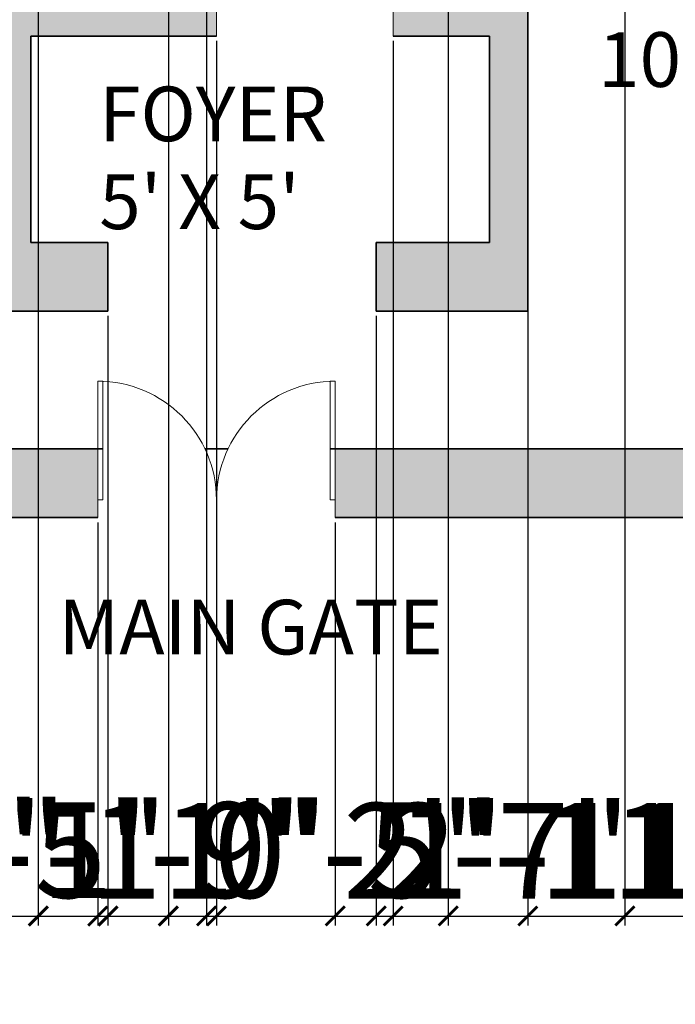
# Model space of a CAD drawing. Units: inches. Extents: x 1763 to 2368, y 1500 to 2097.
# Tile 3 of 24: x 1994 to 2079, y 1500 to 1628. Entities that reach past the tile are written whole.
import ezdxf

# ---------------------------------------------------------------- set-up
doc = ezdxf.new("R2010")
doc.units = ezdxf.units.IN
for name, color, linetype, lineweight in [('A-ANNO-DIMS', 2, 'Continuous', 18), ('A-ANNO-TEXT', 7, 'Continuous', 18), ('A-AREA-IDEN', 7, 'Continuous', 18), ('A-DOOR', 4, 'Continuous', 18), ('A-WALL', 7, 'Continuous', 35), ('A-WALL-PATT', 7, 'Continuous', 13)]:
    doc.layers.add(name, color=color, linetype=linetype, lineweight=lineweight)
doc.styles.get("Standard").update_dxf_attribs({"font": 'arial.ttf'})
doc.dimstyles.new('ISO-25', dxfattribs={"dimtxt": 12.5, "dimasz": 2.5, "dimexe": 1.25, "dimexo": 0.625, "dimtad": 1, "dimdec": 0, "dimlunit": 4, "dimtxsty": 'Standard', "dimblk": 'ARCHTICK', "dimcen": 2.5, "dimclrd": 3, "dimclrt": 4, "dimadec": 0, "dimazin": 0, "dimtfac": 1, "dimtdec": 0, "dimtmove": 0, "dimatfit": 3, "dimfxl": 1, "dimarcsym": 0})

# ---------------------------------------------------------------- blocks, each defined once
blk = doc.blocks.new('*U3')
for p, q in [((0, 0), (0, -6)), ((40, 0), (40, -6))]:
    blk.add_line(p, q)
blk.add_lwpolyline([(0, 0), (0, 40), (1.75, 40), (1.75, 0)], close=True)
blk.add_arc((0, 0), 40, 0, 90)
blk = doc.blocks.new('_ArchTick')
at = {"color": 0, "linetype": 'ByBlock', "const_width": 0.15}
blk.add_lwpolyline([(-0.5, -0.5), (0.5, 0.5)], dxfattribs=at)
blk = doc.blocks.new('*D39')
at = {"layer": 'A-ANNO-DIMS', "color": 0, "lineweight": -2, "transparency": 16777216}
for p, q in [((1829.09, 1562.65), (1829.09, 1509.91)), ((2003.86, 1562.65), (2003.86, 1509.91))]:
    blk.add_line(p, q, dxfattribs=at)
at = {"layer": 'A-ANNO-DIMS', "color": 3, "lineweight": -2, "transparency": 16777216}
blk.add_line((1829.09, 1511.16), (2003.86, 1511.16), dxfattribs=at)
at = {"layer": 'Defpoints', "color": 0, "transparency": 16777216}
for p in [(1829.09, 1563.27), (2003.86, 1563.27), (2003.86, 1511.16)]:
    blk.add_point(p, dxfattribs=at)
at = {"layer": 'A-ANNO-DIMS', "color": 3, "lineweight": -2, "transparency": 16777216, "xscale": 2.5, "yscale": 2.5, "zscale": 2.5, "rotation": 180}
blk.add_blockref('_ArchTick', (1829.09, 1511.16), dxfattribs=at)
at = {"layer": 'A-ANNO-DIMS', "color": 3, "lineweight": -2, "transparency": 16777216, "xscale": 2.5, "yscale": 2.5, "zscale": 2.5}
blk.add_blockref('_ArchTick', (2003.86, 1511.16), dxfattribs=at)
at = {"layer": 'A-ANNO-DIMS', "color": 4, "transparency": 16777216, "insert": (1916.48, 1518.06), "char_height": 12.5, "attachment_point": 5}
blk.add_mtext('14\'-7"', dxfattribs=at)
blk = doc.blocks.new('*D40')
at = {"layer": 'A-ANNO-DIMS', "color": 0, "lineweight": -2, "transparency": 16777216}
for p, q in [((2003.86, 1562.65), (2003.86, 1509.91)), ((2034.91, 1562.65), (2034.91, 1509.91))]:
    blk.add_line(p, q, dxfattribs=at)
at = {"layer": 'A-ANNO-DIMS', "color": 3, "lineweight": -2, "transparency": 16777216}
for p, q in [((2003.86, 1511.16), (2034.91, 1511.16)), ((2034.91, 1511.16), (2072.1, 1511.16))]:
    blk.add_line(p, q, dxfattribs=at)
at = {"layer": 'Defpoints', "color": 0, "transparency": 16777216}
for p in [(2003.86, 1563.27), (2034.91, 1563.27), (2034.91, 1511.16)]:
    blk.add_point(p, dxfattribs=at)
at = {"layer": 'A-ANNO-DIMS', "color": 3, "lineweight": -2, "transparency": 16777216, "xscale": 2.5, "yscale": 2.5, "zscale": 2.5, "rotation": 180}
blk.add_blockref('_ArchTick', (2003.86, 1511.16), dxfattribs=at)
at = {"layer": 'A-ANNO-DIMS', "color": 3, "lineweight": -2, "transparency": 16777216, "xscale": 2.5, "yscale": 2.5, "zscale": 2.5}
blk.add_blockref('_ArchTick', (2034.91, 1511.16), dxfattribs=at)
at = {"layer": 'A-ANNO-DIMS', "color": 4, "transparency": 16777216, "insert": (2054.75, 1518.06), "char_height": 12.5, "attachment_point": 5}
blk.add_mtext('2\'-7"', dxfattribs=at)
blk = doc.blocks.new('*D43')
at = {"layer": 'A-ANNO-DIMS', "color": 0, "lineweight": -2, "transparency": 16777216}
for p, q in [((2060.09, 1589.65), (2060.09, 1509.91)), ((2180.09, 1571.65), (2180.09, 1509.91))]:
    blk.add_line(p, q, dxfattribs=at)
at = {"layer": 'A-ANNO-DIMS', "color": 3, "lineweight": -2, "transparency": 16777216}
blk.add_line((2060.09, 1511.16), (2180.09, 1511.16), dxfattribs=at)
at = {"layer": 'Defpoints', "color": 0, "transparency": 16777216}
for p in [(2060.09, 1590.27), (2180.09, 1572.27), (2180.09, 1511.16)]:
    blk.add_point(p, dxfattribs=at)
at = {"layer": 'A-ANNO-DIMS', "color": 3, "lineweight": -2, "transparency": 16777216, "xscale": 2.5, "yscale": 2.5, "zscale": 2.5, "rotation": 180}
blk.add_blockref('_ArchTick', (2060.09, 1511.16), dxfattribs=at)
at = {"layer": 'A-ANNO-DIMS', "color": 3, "lineweight": -2, "transparency": 16777216, "xscale": 2.5, "yscale": 2.5, "zscale": 2.5}
blk.add_blockref('_ArchTick', (2180.09, 1511.16), dxfattribs=at)
at = {"layer": 'A-ANNO-DIMS', "color": 4, "transparency": 16777216, "insert": (2120.09, 1518.16), "char_height": 12.5, "attachment_point": 5}
blk.add_mtext('10\'-0"', dxfattribs=at)
blk = doc.blocks.new('*D59')
at = {"layer": 'A-ANNO-DIMS', "color": 0, "lineweight": -2, "transparency": 16777216}
for p, q in [((2019.39, 1625.65), (2019.39, 1509.91)), ((2042.48, 1625.65), (2042.48, 1509.91))]:
    blk.add_line(p, q, dxfattribs=at)
at = {"layer": 'A-ANNO-DIMS', "color": 3, "lineweight": -2, "transparency": 16777216}
for p, q in [((2019.39, 1511.16), (2042.48, 1511.16)), ((2042.48, 1511.16), (2088, 1511.16))]:
    blk.add_line(p, q, dxfattribs=at)
at = {"layer": 'Defpoints', "color": 0, "transparency": 16777216}
for p in [(2019.39, 1626.27), (2042.48, 1626.27), (2042.48, 1511.16)]:
    blk.add_point(p, dxfattribs=at)
at = {"layer": 'A-ANNO-DIMS', "color": 3, "lineweight": -2, "transparency": 16777216, "xscale": 2.5, "yscale": 2.5, "zscale": 2.5, "rotation": 180}
blk.add_blockref('_ArchTick', (2019.39, 1511.16), dxfattribs=at)
at = {"layer": 'A-ANNO-DIMS', "color": 3, "lineweight": -2, "transparency": 16777216, "xscale": 2.5, "yscale": 2.5, "zscale": 2.5}
blk.add_blockref('_ArchTick', (2042.48, 1511.16), dxfattribs=at)
at = {"layer": 'A-ANNO-DIMS', "color": 4, "transparency": 16777216, "insert": (2066.49, 1518.06), "char_height": 12.5, "attachment_point": 5}
blk.add_mtext('1\'-11"', dxfattribs=at)
blk = doc.blocks.new('*D60')
at = {"layer": 'A-ANNO-DIMS', "color": 0, "lineweight": -2, "transparency": 16777216}
for p, q in [((2060.09, 1678.65), (2060.09, 1509.91)), ((2100.58, 1678.65), (2100.58, 1509.91))]:
    blk.add_line(p, q, dxfattribs=at)
at = {"layer": 'A-ANNO-DIMS', "color": 3, "lineweight": -2, "transparency": 16777216}
for p, q in [((2060.09, 1511.16), (2100.58, 1511.16)), ((2100.58, 1511.16), (2166.67, 1511.16))]:
    blk.add_line(p, q, dxfattribs=at)
at = {"layer": 'Defpoints', "color": 0, "transparency": 16777216}
for p in [(2060.09, 1679.27), (2100.58, 1679.27), (2100.58, 1511.16)]:
    blk.add_point(p, dxfattribs=at)
at = {"layer": 'A-ANNO-DIMS', "color": 3, "lineweight": -2, "transparency": 16777216, "xscale": 2.5, "yscale": 2.5, "zscale": 2.5, "rotation": 180}
blk.add_blockref('_ArchTick', (2060.09, 1511.16), dxfattribs=at)
at = {"layer": 'A-ANNO-DIMS', "color": 3, "lineweight": -2, "transparency": 16777216, "xscale": 2.5, "yscale": 2.5, "zscale": 2.5}
blk.add_blockref('_ArchTick', (2100.58, 1511.16), dxfattribs=at)
at = {"layer": 'A-ANNO-DIMS', "color": 4, "transparency": 16777216, "insert": (2134.88, 1518.25), "char_height": 12.5, "attachment_point": 5}
blk.add_mtext('3\'-4 1/2"', dxfattribs=at)
blk = doc.blocks.new('*D68')
at = {"layer": 'A-ANNO-DIMS', "color": 0, "lineweight": -2, "transparency": 16777216}
for p, q in [((1895.59, 1879.65), (1895.59, 1509.91)), ((1932.01, 1879.65), (1932.01, 1509.91))]:
    blk.add_line(p, q, dxfattribs=at)
at = {"layer": 'A-ANNO-DIMS', "color": 3, "lineweight": -2, "transparency": 16777216}
for p, q in [((1895.59, 1511.16), (1932.01, 1511.16)), ((1932.01, 1511.16), (1998.11, 1511.16))]:
    blk.add_line(p, q, dxfattribs=at)
at = {"layer": 'Defpoints', "color": 0, "transparency": 16777216}
for p in [(1895.59, 1880.27), (1932.01, 1880.27), (1932.01, 1511.16)]:
    blk.add_point(p, dxfattribs=at)
at = {"layer": 'A-ANNO-DIMS', "color": 3, "lineweight": -2, "transparency": 16777216, "xscale": 2.5, "yscale": 2.5, "zscale": 2.5, "rotation": 180}
blk.add_blockref('_ArchTick', (1895.59, 1511.16), dxfattribs=at)
at = {"layer": 'A-ANNO-DIMS', "color": 3, "lineweight": -2, "transparency": 16777216, "xscale": 2.5, "yscale": 2.5, "zscale": 2.5}
blk.add_blockref('_ArchTick', (1932.01, 1511.16), dxfattribs=at)
at = {"layer": 'A-ANNO-DIMS', "color": 4, "transparency": 16777216, "insert": (1966.31, 1518.25), "char_height": 12.5, "attachment_point": 5}
blk.add_mtext('3\'-0 1/2"', dxfattribs=at)
blk = doc.blocks.new('*D70')
at = {"layer": 'A-ANNO-DIMS', "color": 0, "lineweight": -2, "transparency": 16777216}
for p, q in [((1959.13, 1879.65), (1959.13, 1509.91)), ((1982.23, 1879.65), (1982.23, 1509.91))]:
    blk.add_line(p, q, dxfattribs=at)
at = {"layer": 'A-ANNO-DIMS', "color": 3, "lineweight": -2, "transparency": 16777216}
for p, q in [((1959.13, 1511.16), (1982.23, 1511.16)), ((1982.23, 1511.16), (2027.75, 1511.16))]:
    blk.add_line(p, q, dxfattribs=at)
at = {"layer": 'Defpoints', "color": 0, "transparency": 16777216}
for p in [(1959.13, 1880.27), (1982.23, 1880.27), (1982.23, 1511.16)]:
    blk.add_point(p, dxfattribs=at)
at = {"layer": 'A-ANNO-DIMS', "color": 3, "lineweight": -2, "transparency": 16777216, "xscale": 2.5, "yscale": 2.5, "zscale": 2.5, "rotation": 180}
blk.add_blockref('_ArchTick', (1959.13, 1511.16), dxfattribs=at)
at = {"layer": 'A-ANNO-DIMS', "color": 3, "lineweight": -2, "transparency": 16777216, "xscale": 2.5, "yscale": 2.5, "zscale": 2.5}
blk.add_blockref('_ArchTick', (1982.23, 1511.16), dxfattribs=at)
at = {"layer": 'A-ANNO-DIMS', "color": 4, "transparency": 16777216, "insert": (2006.24, 1518.06), "char_height": 12.5, "attachment_point": 5}
blk.add_mtext('1\'-11"', dxfattribs=at)
blk = doc.blocks.new('*D71')
at = {"layer": 'A-ANNO-DIMS', "color": 0, "lineweight": -2, "transparency": 16777216}
for p, q in [((2049.69, 1879.65), (2049.69, 1509.91)), ((2072.78, 1879.65), (2072.78, 1509.91))]:
    blk.add_line(p, q, dxfattribs=at)
at = {"layer": 'A-ANNO-DIMS', "color": 3, "lineweight": -2, "transparency": 16777216}
for p, q in [((2049.69, 1511.16), (2072.78, 1511.16)), ((2072.78, 1511.16), (2118.3, 1511.16))]:
    blk.add_line(p, q, dxfattribs=at)
at = {"layer": 'Defpoints', "color": 0, "transparency": 16777216}
for p in [(2049.69, 1880.27), (2072.78, 1880.27), (2072.78, 1511.16)]:
    blk.add_point(p, dxfattribs=at)
at = {"layer": 'A-ANNO-DIMS', "color": 3, "lineweight": -2, "transparency": 16777216, "xscale": 2.5, "yscale": 2.5, "zscale": 2.5, "rotation": 180}
blk.add_blockref('_ArchTick', (2049.69, 1511.16), dxfattribs=at)
at = {"layer": 'A-ANNO-DIMS', "color": 3, "lineweight": -2, "transparency": 16777216, "xscale": 2.5, "yscale": 2.5, "zscale": 2.5}
blk.add_blockref('_ArchTick', (2072.78, 1511.16), dxfattribs=at)
at = {"layer": 'A-ANNO-DIMS', "color": 4, "transparency": 16777216, "insert": (2096.79, 1518.06), "char_height": 12.5, "attachment_point": 5}
blk.add_mtext('1\'-11"', dxfattribs=at)
blk = doc.blocks.new('*D77')
at = {"layer": 'A-ANNO-DIMS', "color": 0, "lineweight": -2, "transparency": 16777216}
for p, q in [((1975.09, 1972.65), (1975.09, 1509.91)), ((1996.09, 1972.65), (1996.09, 1509.91))]:
    blk.add_line(p, q, dxfattribs=at)
at = {"layer": 'A-ANNO-DIMS', "color": 3, "lineweight": -2, "transparency": 16777216}
for p, q in [((1975.09, 1511.16), (1996.09, 1511.16)), ((1996.09, 1511.16), (2031.89, 1511.16))]:
    blk.add_line(p, q, dxfattribs=at)
at = {"layer": 'Defpoints', "color": 0, "transparency": 16777216}
for p in [(1975.09, 1973.27), (1996.09, 1973.27), (1996.09, 1511.16)]:
    blk.add_point(p, dxfattribs=at)
at = {"layer": 'A-ANNO-DIMS', "color": 3, "lineweight": -2, "transparency": 16777216, "xscale": 2.5, "yscale": 2.5, "zscale": 2.5, "rotation": 180}
blk.add_blockref('_ArchTick', (1975.09, 1511.16), dxfattribs=at)
at = {"layer": 'A-ANNO-DIMS', "color": 3, "lineweight": -2, "transparency": 16777216, "xscale": 2.5, "yscale": 2.5, "zscale": 2.5}
blk.add_blockref('_ArchTick', (1996.09, 1511.16), dxfattribs=at)
at = {"layer": 'A-ANNO-DIMS', "color": 4, "transparency": 16777216, "insert": (2015.24, 1518.16), "char_height": 12.5, "attachment_point": 5}
blk.add_mtext('1\'-9"', dxfattribs=at)
blk = doc.blocks.new('*D83')
at = {"layer": 'A-ANNO-DIMS', "color": 0, "lineweight": -2, "transparency": 16777216}
for p, q in [((2005.2, 1589.65), (2005.2, 1509.91)), ((2040.27, 1589.65), (2040.27, 1509.91))]:
    blk.add_line(p, q, dxfattribs=at)
at = {"layer": 'A-ANNO-DIMS', "color": 3, "lineweight": -2, "transparency": 16777216}
for p, q in [((2005.2, 1511.16), (2040.27, 1511.16)), ((2040.27, 1511.16), (2087.17, 1511.16))]:
    blk.add_line(p, q, dxfattribs=at)
at = {"layer": 'Defpoints', "color": 0, "transparency": 16777216}
for p in [(2005.2, 1590.27), (2040.27, 1590.27), (2040.27, 1511.16)]:
    blk.add_point(p, dxfattribs=at)
at = {"layer": 'A-ANNO-DIMS', "color": 3, "lineweight": -2, "transparency": 16777216, "xscale": 2.5, "yscale": 2.5, "zscale": 2.5, "rotation": 180}
blk.add_blockref('_ArchTick', (2005.2, 1511.16), dxfattribs=at)
at = {"layer": 'A-ANNO-DIMS', "color": 3, "lineweight": -2, "transparency": 16777216, "xscale": 2.5, "yscale": 2.5, "zscale": 2.5}
blk.add_blockref('_ArchTick', (2040.27, 1511.16), dxfattribs=at)
at = {"layer": 'A-ANNO-DIMS', "color": 4, "transparency": 16777216, "insert": (2064.97, 1518.06), "char_height": 12.5, "attachment_point": 5}
blk.add_mtext('2\'-11"', dxfattribs=at)
blk = doc.blocks.new('*D86')
at = {"layer": 'A-ANNO-DIMS', "color": 0, "lineweight": -2, "transparency": 16777216}
for p, q in [((2013.09, 1884.65), (2013.09, 1509.91)), ((2018.09, 1884.65), (2018.09, 1509.91))]:
    blk.add_line(p, q, dxfattribs=at)
at = {"layer": 'A-ANNO-DIMS', "color": 3, "lineweight": -2, "transparency": 16777216}
for p, q in [((2013.09, 1511.16), (2018.09, 1511.16)), ((2018.09, 1511.16), (2055.07, 1511.16))]:
    blk.add_line(p, q, dxfattribs=at)
at = {"layer": 'Defpoints', "color": 0, "transparency": 16777216}
for p in [(2013.09, 1885.27), (2018.09, 1885.27), (2018.09, 1511.16)]:
    blk.add_point(p, dxfattribs=at)
at = {"layer": 'A-ANNO-DIMS', "color": 3, "lineweight": -2, "transparency": 16777216, "xscale": 2.5, "yscale": 2.5, "zscale": 2.5, "rotation": 180}
blk.add_blockref('_ArchTick', (2013.09, 1511.16), dxfattribs=at)
at = {"layer": 'A-ANNO-DIMS', "color": 3, "lineweight": -2, "transparency": 16777216, "xscale": 2.5, "yscale": 2.5, "zscale": 2.5}
blk.add_blockref('_ArchTick', (2018.09, 1511.16), dxfattribs=at)
at = {"layer": 'A-ANNO-DIMS', "color": 4, "transparency": 16777216, "insert": (2037.83, 1518.16), "char_height": 12.5, "attachment_point": 5}
blk.add_mtext('0\'-5"', dxfattribs=at)
blk = doc.blocks.new('*D87')
at = {"layer": 'A-ANNO-DIMS', "color": 0, "lineweight": -2, "transparency": 16777216}
for p, q in [((1958.09, 1980.65), (1958.09, 1509.91)), ((1975.09, 1980.65), (1975.09, 1509.91))]:
    blk.add_line(p, q, dxfattribs=at)
at = {"layer": 'A-ANNO-DIMS', "color": 3, "lineweight": -2, "transparency": 16777216}
for p, q in [((1958.09, 1511.16), (1975.09, 1511.16)), ((1975.09, 1511.16), (2010.89, 1511.16))]:
    blk.add_line(p, q, dxfattribs=at)
at = {"layer": 'Defpoints', "color": 0, "transparency": 16777216}
for p in [(1958.09, 1981.27), (1975.09, 1981.27), (1975.09, 1511.16)]:
    blk.add_point(p, dxfattribs=at)
at = {"layer": 'A-ANNO-DIMS', "color": 3, "lineweight": -2, "transparency": 16777216, "xscale": 2.5, "yscale": 2.5, "zscale": 2.5, "rotation": 180}
blk.add_blockref('_ArchTick', (1958.09, 1511.16), dxfattribs=at)
at = {"layer": 'A-ANNO-DIMS', "color": 3, "lineweight": -2, "transparency": 16777216, "xscale": 2.5, "yscale": 2.5, "zscale": 2.5}
blk.add_blockref('_ArchTick', (1975.09, 1511.16), dxfattribs=at)
at = {"layer": 'A-ANNO-DIMS', "color": 4, "transparency": 16777216, "insert": (1994.24, 1518.16), "char_height": 12.5, "attachment_point": 5}
blk.add_mtext('1\'-5"', dxfattribs=at)

msp = doc.modelspace()

# ---------------------------------------------------------------- hatches: boundary and pattern name
at = {"layer": 'A-WALL-PATT'}
h = msp.add_hatch(color=256, dxfattribs=at)
h.dxf.hatch_style = 1
h.paths.add_polyline_path([(1838.09, 2034.27), (1838.09, 2043.27), (1829.09, 2043.27), (1829.09, 1953.39), (1838.09, 1953.39)])
h.paths.add_polyline_path([(1838.09, 1913.1), (1829.09, 1913.1), (1829.09, 1862.2), (1838.09, 1862.2)])
h.paths.add_polyline_path([(1838.09, 1825.59), (1829.09, 1825.59), (1829.09, 1738.64), (1838.09, 1738.64)])
h.paths.add_polyline_path([(1895.59, 1885.27), (1838.09, 1885.27), (1838.09, 1880.27), (1895.59, 1880.27)])
h.paths.add_polyline_path([(1857.39, 1784.27), (1838.09, 1784.27), (1838.09, 1779.27), (1857.39, 1779.27)])
h.paths.add_polyline_path([(1958.09, 1981.27), (1971.46, 1981.27), (1971.46, 1986.27), (1968.57, 1986.27), (1958.09, 1986.27), (1953.09, 1986.27), (1927.39, 1986.27), (1927.39, 1981.27), (1953.09, 1981.27), (1953.09, 1885.27), (1932.01, 1885.27), (1932.01, 1880.27), (1959.13, 1880.27), (1959.13, 1883.74), (1959.13, 1885.27), (1958.09, 1885.27)])
h.paths.add_polyline_path([(2018.09, 1981.27), (2031.02, 1981.27), (2031.02, 1986.27), (2018.09, 1986.27), (2013.09, 1986.27), (2001.23, 1986.27), (2001.23, 1981.27), (2013.09, 1981.27), (2013.09, 1885.27), (1982.18, 1885.27, -0.016629), (1982.23, 1883.74), (1982.23, 1880.27), (2049.69, 1880.27), (2049.69, 1883.74, -0.016629), (2049.74, 1885.27), (2018.09, 1885.27)])
h.paths.add_polyline_path([(2083.09, 1981.27), (2120.61, 1981.27), (2120.61, 1986.27), (2083.09, 1986.27), (2078.09, 1986.27), (2063.14, 1986.27), (2063.14, 1981.27), (2078.09, 1981.27), (2078.09, 1885.27), (2072.78, 1885.27), (2072.78, 1883.74), (2072.78, 1880.27), (2078.09, 1880.27), (2078.09, 1866.87), (2081.56, 1866.87, -0.016629), (2083.09, 1866.82)])
h.paths.add_polyline_path([(1871.68, 1635.27), (1838.09, 1635.27), (1838.09, 1626.27), (1871.68, 1626.27)], flags=17)
h.paths.add_polyline_path([(2100.58, 1688.27), (2060.09, 1688.27), (2060.09, 1679.27), (2100.58, 1679.27)], flags=17)
h.paths.add_polyline_path([(2180.09, 1688.27), (2148.74, 1688.27), (2148.74, 1679.27), (2180.09, 1679.27)], flags=17)
h.paths.add_polyline_path([(2189.09, 1746.22), (2180.09, 1746.22), (2180.09, 1743.42), (2180.12, 1743.42), (2180.12, 1726.72), (2180.09, 1572.27), (2034.91, 1572.27), (2034.91, 1565.6), (2034.91, 1563.27), (2189.09, 1563.27)])
h.paths.add_polyline_path([(2060.09, 1802.35, -0.016629), (2058.56, 1802.3), (2055.09, 1802.3), (2055.09, 1635.27), (2042.48, 1635.27), (2042.48, 1629.74), (2042.48, 1626.27), (2055.09, 1626.27), (2055.09, 1599.27), (2040.27, 1599.27), (2040.27, 1590.27), (2060.09, 1590.27)])
h.paths.add_polyline_path([(2019.39, 1629.74, -0.060569), (2020.06, 1635.27), (1995.09, 1635.27), (1990.09, 1635.27), (1927.07, 1635.27), (1927.07, 1626.27), (1990.09, 1626.27), (1990.09, 1590.27), (1995.09, 1590.27), (2005.2, 1590.27), (2005.2, 1599.27), (1995.09, 1599.27), (1995.09, 1626.27), (2019.39, 1626.27)])
edge = h.paths.add_edge_path()
edge.add_line((2180.09, 1837.27), (2167.2, 1837.27))
edge.add_spline(control_points=[(2167.2, 1837.27), (2167.19, 1837.27), (2167.18, 1837.27), (2167.18, 1837.27)], knot_values=[168.955493, 168.955493, 168.955493, 168.955493, 169.065871, 169.065871, 169.065871, 169.065871], degree=3, periodic=0)
edge.add_spline(control_points=[(2167.18, 1837.27), (2166.56, 1837.38), (2166.33, 1846.16), (2165.71, 1846.24)], knot_values=[159.864705, 159.864705, 159.864705, 159.864705, 168.955493, 168.955493, 168.955493, 168.955493], degree=3, periodic=0)
edge.add_line((2167.12, 1837.27), (2163.16, 1837.27))
edge.add_spline(control_points=[(2163.16, 1837.27), (2163.16, 1837.27), (2163.16, 1837.27), (2163.15, 1837.27)], knot_values=[150.537172, 150.537172, 150.537172, 150.537172, 150.553797, 150.553797, 150.553797, 150.553797], degree=3, periodic=0)
edge.add_spline(control_points=[(2163.15, 1837.27), (2162.29, 1837.29), (2161.59, 1846.23), (2160.88, 1846.24)], knot_values=[141.293426, 141.293426, 141.293426, 141.293426, 150.537172, 150.537172, 150.537172, 150.537172], degree=3, periodic=0)
edge.add_line((2163.08, 1837.27), (2158.7, 1837.27))
edge.add_spline(control_points=[(2158.7, 1837.27), (2158.7, 1837.27), (2158.7, 1837.27), (2158.7, 1837.27)], knot_values=[132.033544, 132.033544, 132.033544, 132.033544, 132.049151, 132.049151, 132.049151, 132.049151], degree=3, periodic=0)
edge.add_spline(control_points=[(2158.7, 1837.27), (2157.97, 1837.29), (2157.26, 1846.23), (2156.39, 1846.24)], knot_values=[122.786021, 122.786021, 122.786021, 122.786021, 132.033544, 132.033544, 132.033544, 132.033544], degree=3, periodic=0)
edge.add_line((2158.63, 1837.27), (2153.84, 1837.27))
edge.add_spline(control_points=[(2153.84, 1837.27), (2153.83, 1837.27), (2153.82, 1837.27), (2153.82, 1837.27)], knot_values=[113.451585, 113.451585, 113.451585, 113.451585, 113.562103, 113.562103, 113.562103, 113.562103], degree=3, periodic=0)
edge.add_spline(control_points=[(2153.82, 1837.27), (2153.17, 1837.38), (2152.88, 1846.19), (2152.4, 1846.24)], knot_values=[0, 0, 0, 0, 9.081854, 9.081854, 9.081854, 9.081854], degree=3, periodic=0)
edge.add_line((2153.76, 1837.27), (2150.39, 1837.27))
edge.add_spline(control_points=[(2150.39, 1837.27), (2150.38, 1837.27), (2150.37, 1837.27), (2150.36, 1837.27)], knot_values=[95.069382, 95.069382, 95.069382, 95.069382, 95.17519, 95.17519, 95.17519, 95.17519], degree=3, periodic=0)
edge.add_spline(control_points=[(2150.36, 1837.27), (2149.49, 1837.37), (2148.42, 1846.19), (2147.59, 1846.24)], knot_values=[85.824599, 85.824599, 85.824599, 85.824599, 95.069382, 95.069382, 95.069382, 95.069382], degree=3, periodic=0)
edge.add_line((2150.29, 1837.27), (2145.43, 1837.27))
edge.add_spline(control_points=[(2145.43, 1837.27), (2145.43, 1837.27), (2145.42, 1837.27), (2145.42, 1837.27)], knot_values=[76.505559, 76.505559, 76.505559, 76.505559, 76.547811, 76.547811, 76.547811, 76.547811], degree=3, periodic=0)
edge.add_spline(control_points=[(2145.42, 1837.27), (2144.68, 1837.31), (2143.8, 1846.19), (2142.95, 1846.24)], knot_values=[67.23945, 67.23945, 67.23945, 67.23945, 76.505559, 76.505559, 76.505559, 76.505559], degree=3, periodic=0)
edge.add_line((2145.35, 1837.27), (2134.57, 1837.27))
edge.add_spline(control_points=[(2134.57, 1837.27), (2134.57, 1837.27), (2134.56, 1837.27), (2134.56, 1837.27)], knot_values=[39.001463, 39.001463, 39.001463, 39.001463, 39.045107, 39.045107, 39.045107, 39.045107], degree=3, periodic=0)
edge.add_spline(control_points=[(2134.56, 1837.27), (2133.87, 1837.31), (2133.4, 1845.85), (2132.33, 1846.24)], knot_values=[29.79778, 29.79778, 29.79778, 29.79778, 39.001463, 39.001463, 39.001463, 39.001463], degree=3, periodic=0)
edge.add_line((2134.5, 1837.27), (2128.08, 1837.27))
edge.add_spline(control_points=[(2128.08, 1837.27), (2128.03, 1837.26), (2127.98, 1837.26), (2127.93, 1837.27)], knot_values=[19.482067, 19.482067, 19.482067, 19.482067, 19.869396, 19.869396, 19.869396, 19.869396], degree=3, periodic=0)
edge.add_spline(control_points=[(2125.01, 1846.24), (2126.16, 1844.66), (2126.82, 1837.57), (2127.93, 1837.27)], knot_values=[10.389805, 10.389805, 10.389805, 10.389805, 19.482067, 19.482067, 19.482067, 19.482067], degree=3, periodic=0)
edge.add_line((2127.93, 1837.27), (2083.09, 1837.27))
edge.add_line((2083.09, 1837.27), (2083.09, 1843.77))
edge.add_line((2083.09, 1843.77), (2081.56, 1843.77))
edge.add_line((2081.56, 1843.77), (2078.09, 1843.77))
edge.add_line((2078.09, 1843.77), (2078.09, 1837.27))
edge.add_line((2078.09, 1837.27), (2055.09, 1837.27))
edge.add_line((2055.09, 1837.27), (2055.09, 1825.4))
edge.add_line((2055.09, 1825.4), (2058.56, 1825.4))
edge.add_line((2058.56, 1825.4), (2060.09, 1825.4))
edge.add_line((2060.09, 1825.4), (2060.09, 1832.27))
edge.add_line((2060.09, 1832.27), (2122.44, 1832.27))
edge.add_spline(control_points=[(2122.44, 1832.27), (2122.73, 1832.58), (2123.01, 1832.62), (2123.28, 1832.27)], knot_values=[5.972033, 5.972033, 5.972033, 5.972033, 8.057258, 8.057258, 8.057258, 8.057258], degree=3, periodic=0)
edge.add_line((2123.28, 1832.27), (2137.95, 1832.27))
edge.add_spline(control_points=[(2137.95, 1832.27), (2137.96, 1832.27), (2137.97, 1832.27), (2137.98, 1832.27)], knot_values=[53.926862, 53.926862, 53.926862, 53.926862, 54.030075, 54.030075, 54.030075, 54.030075], degree=3, periodic=0)
edge.add_spline(control_points=[(2139.72, 1825.02), (2139.28, 1825.06), (2138.67, 1832.18), (2137.98, 1832.27)], knot_values=[54.030075, 54.030075, 54.030075, 54.030075, 61.445194, 61.445194, 61.445194, 61.445194], degree=3, periodic=0)
edge.add_line((2138.05, 1832.27), (2140.96, 1832.27))
edge.add_spline(control_points=[(2140.96, 1832.27), (2140.97, 1832.27), (2140.98, 1832.27), (2140.99, 1832.27)], knot_values=[68.854182, 68.854182, 68.854182, 68.854182, 68.971237, 68.971237, 68.971237, 68.971237], degree=3, periodic=0)
edge.add_spline(control_points=[(2143.19, 1825.02), (2142.44, 1825.07), (2141.56, 1832.16), (2140.99, 1832.27)], knot_values=[68.971237, 68.971237, 68.971237, 68.971237, 76.444911, 76.444911, 76.444911, 76.444911], degree=3, periodic=0)
edge.add_line((2141.04, 1832.27), (2145.43, 1832.27))
edge.add_spline(control_points=[(2145.43, 1832.27), (2145.44, 1832.27), (2145.45, 1832.27), (2145.46, 1832.27)], knot_values=[84.039047, 84.039047, 84.039047, 84.039047, 84.124041, 84.124041, 84.124041, 84.124041], degree=3, periodic=0)
edge.add_spline(control_points=[(2148.11, 1825.02), (2147.34, 1825.02), (2146.3, 1832.19), (2145.46, 1832.27)], knot_values=[84.124041, 84.124041, 84.124041, 84.124041, 91.773891, 91.773891, 91.773891, 91.773891], degree=3, periodic=0)
edge.add_line((2145.54, 1832.27), (2150.39, 1832.27))
edge.add_spline(control_points=[(2150.39, 1832.27), (2150.42, 1832.28), (2150.45, 1832.28), (2150.47, 1832.27)], knot_values=[99.381577, 99.381577, 99.381577, 99.381577, 99.573457, 99.573457, 99.573457, 99.573457], degree=3, periodic=0)
edge.add_spline(control_points=[(2153.97, 1825.02), (2153.09, 1825.28), (2151.53, 1832.1), (2150.47, 1832.27)], knot_values=[99.573457, 99.573457, 99.573457, 99.573457, 107.218357, 107.218357, 107.218357, 107.218357], degree=3, periodic=0)
edge.add_line((2150.57, 1832.27), (2155.6, 1832.27))
edge.add_spline(control_points=[(2155.6, 1832.27), (2155.6, 1832.27), (2155.61, 1832.27), (2155.62, 1832.27)], knot_values=[114.933058, 114.933058, 114.933058, 114.933058, 115.013624, 115.013624, 115.013624, 115.013624], degree=3, periodic=0)
edge.add_spline(control_points=[(2158.28, 1825.02), (2157.4, 1825.07), (2156.25, 1832.2), (2155.62, 1832.27)], knot_values=[115.013624, 115.013624, 115.013624, 115.013624, 122.616269, 122.616269, 122.616269, 122.616269], degree=3, periodic=0)
edge.add_line((2155.68, 1832.27), (2165.19, 1832.27))
edge.add_spline(control_points=[(2165.19, 1832.27), (2165.2, 1832.27), (2165.2, 1832.27), (2165.2, 1832.27)], knot_values=[145.488477, 145.488477, 145.488477, 145.488477, 145.516379, 145.516379, 145.516379, 145.516379], degree=3, periodic=0)
edge.add_spline(control_points=[(2167.45, 1825.02), (2166.96, 1825.02), (2166.06, 1832.25), (2165.2, 1832.27)], knot_values=[145.516379, 145.516379, 145.516379, 145.516379, 153.105469, 153.105469, 153.105469, 153.105469], degree=3, periodic=0)
edge.add_line((2165.29, 1832.27), (2168.93, 1832.27))
edge.add_spline(control_points=[(2168.93, 1832.27), (2168.98, 1832.29), (2169.04, 1832.29), (2169.1, 1832.27)], knot_values=[160.517439, 160.517439, 160.517439, 160.517439, 160.939723, 160.939723, 160.939723, 160.939723], degree=3, periodic=0)
edge.add_spline(control_points=[(2171.09, 1828.64), (2170.35, 1830.37), (2169.62, 1832.09), (2169.1, 1832.27)], knot_values=[160.939723, 160.939723, 160.939723, 160.939723, 164.738835, 164.738835, 164.738835, 164.738835], degree=3, periodic=0)
edge.add_line((2169.1, 1832.27), (2180.09, 1832.27))
edge.add_line((2180.09, 1832.27), (2180.09, 1837.27))
h.paths.add_polyline_path([(2189.09, 1885.52), (2180.09, 1885.52), (2180.09, 1813.32), (2180.12, 1813.32), (2180.12, 1796.62), (2180.12, 1795.26), (2189.09, 1795.26)])
h.paths.add_polyline_path([(2180.09, 1986.27), (2166.28, 1986.27), (2166.28, 1981.27), (2180.09, 1981.27)])
h.paths.add_polyline_path([(2189.09, 2043.27), (2180.09, 2043.27), (2180.09, 2034.27), (2180.09, 1934.11), (2189.09, 1934.11)])
h.paths.add_polyline_path([(1838.09, 1681.59), (1829.09, 1681.59), (1829.09, 1563.27), (2003.86, 1563.27), (2003.86, 1565.6), (2003.86, 1572.27), (1838.09, 1572.27)])

# ---------------------------------------------------------------- linework, layer by layer
at = {"layer": 'A-WALL'}
for p, q in [((2060.09, 1802.35), (2060.09, 1590.27)), ((1995.09, 1626.27), (1995.09, 1599.27)), ((1995.09, 1626.27), (2019.39, 1626.27)), ((2042.48, 1626.27), (2055.09, 1626.27)), ((2055.09, 1626.27), (2055.09, 1599.27)), ((1995.09, 1599.27), (2005.2, 1599.27)), ((2005.2, 1599.27), (2005.2, 1590.27)), ((2040.27, 1599.27), (2040.27, 1590.27)), ((2040.27, 1599.27), (2055.09, 1599.27)), ((1995.09, 1590.27), (1990.09, 1590.27)), ((1995.09, 1590.27), (2005.2, 1590.27)), ((2040.27, 1590.27), (2060.09, 1590.27)), ((2004.54, 1572.27), (1838.09, 1572.27)), ((2020.89, 1572.27), (2017.88, 1572.27)), ((2180.09, 1572.27), (2034.23, 1572.27))]:
    msp.add_line(p, q, dxfattribs=at)
msp.add_lwpolyline([(2003.86, 1563.27), (1829.09, 1563.27), (1829.09, 2043.27), (2189.09, 2043.27), (2189.09, 1563.27), (2034.91, 1563.27)], dxfattribs=at)

# ---------------------------------------------------------------- block references
at = {"layer": 'A-DOOR'}
for p, xscale, yscale, zscale in [((2042.48, 1629.74), -0.5774759422388936, 0.5774759422388936, 0.5774759422388936), ((2003.86, 1565.6), 0.3880339817319647, 0.3880339817319647, 0.3880339817319647), ((2034.91, 1565.6), -0.3880339817319647, 0.3880339817319647, 0.3880339817319647)]:
    msp.add_blockref('*U3', p, dxfattribs=dict(at, xscale=xscale, yscale=yscale, zscale=zscale))

# ---------------------------------------------------------------- texts
at = {"layer": 'A-ANNO-TEXT'}
msp.add_text('MAIN GATE', height=7.155, dxfattribs=at).set_placement((1998.74, 1545.37))
at = {"layer": 'A-AREA-IDEN'}
for s, p in [('10\'6"X16\'', (2069.29, 1619.62)), ('FOYER', (2004.06, 1612.51)), ("5' X 5'", (2004.06, 1601.02))]:
    msp.add_text(s, height=7.155, dxfattribs=at).set_placement(p)

# ---------------------------------------------------------------- dimensions: what is measured, and where the dimension line sits
at = {"layer": 'A-ANNO-DIMS'}
for base, p1, p2, picture, middle in [((1975.09, 1511.16), (1958.09, 1981.27), (1975.09, 1981.27), '*D87', (1994.24, 1518.16)), ((1996.09, 1511.16), (1975.09, 1973.27), (1996.09, 1973.27), '*D77', (2015.24, 1518.16)), ((2018.09, 1511.16), (2013.09, 1885.27), (2018.09, 1885.27), '*D86', (2037.83, 1518.16)), ((1932.01, 1511.16), (1895.59, 1880.27), (1932.01, 1880.27), '*D68', (1966.31, 1518.25)), ((1982.23, 1511.16), (1959.13, 1880.27), (1982.23, 1880.27), '*D70', (2006.24, 1518.06)), ((2072.78, 1511.16), (2049.69, 1880.27), (2072.78, 1880.27), '*D71', (2096.79, 1518.06)), ((2100.58, 1511.16), (2060.09, 1679.27), (2100.58, 1679.27), '*D60', (2134.88, 1518.25)), ((2042.48, 1511.16), (2019.39, 1626.27), (2042.48, 1626.27), '*D59', (2066.49, 1518.06)), ((2040.27, 1511.16), (2005.2, 1590.27), (2040.27, 1590.27), '*D83', (2064.97, 1518.06)), ((2180.09, 1511.16), (2060.09, 1590.27), (2180.09, 1572.27), '*D43', (2120.09, 1518.16)), ((2003.86, 1511.16), (1829.09, 1563.27), (2003.86, 1563.27), '*D39', (1916.48, 1518.06)), ((2034.9068, 1511.1561), (2003.8641, 1563.2727), (2034.9068, 1563.2727), '*D40', (2054.7525, 1518.0567))]:
    dim = msp.add_linear_dim(base=base, p1=p1, p2=p2, dimstyle='ISO-25', override={"dimdec": 1, "dimlfac": 1, "dimrnd": 0, "dimzin": 1, "dimdsep": 46, "dimlunit": 4, "dimfrac": 2}, dxfattribs=at)
    dim.commit()
    dim.dimension.update_dxf_attribs({"geometry": picture, "text_midpoint": middle})

doc.saveas('drawing.dxf')
